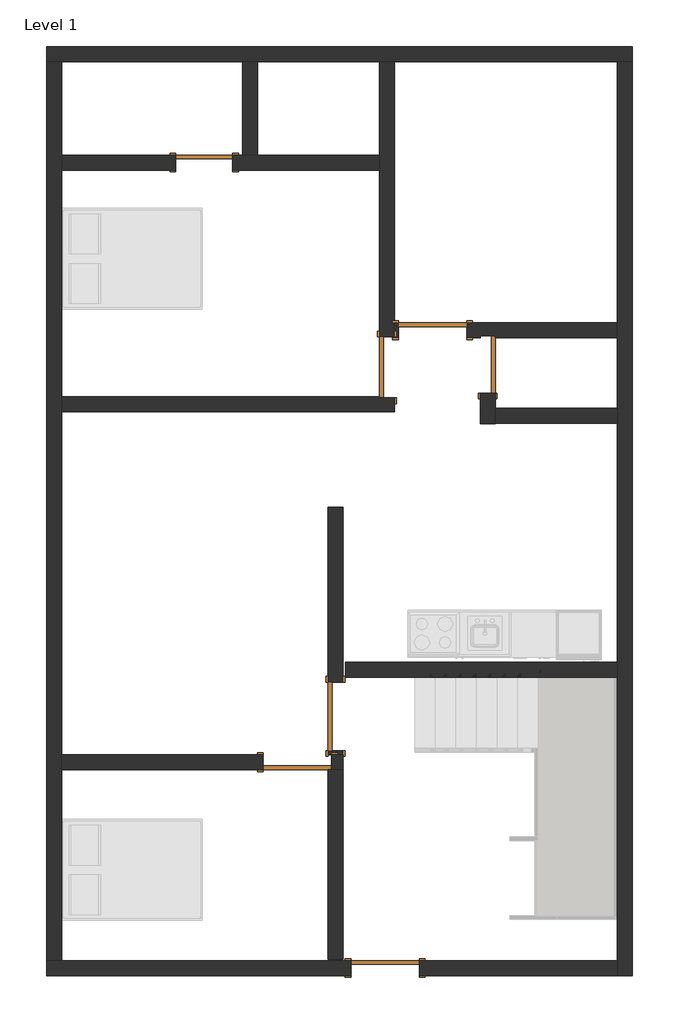
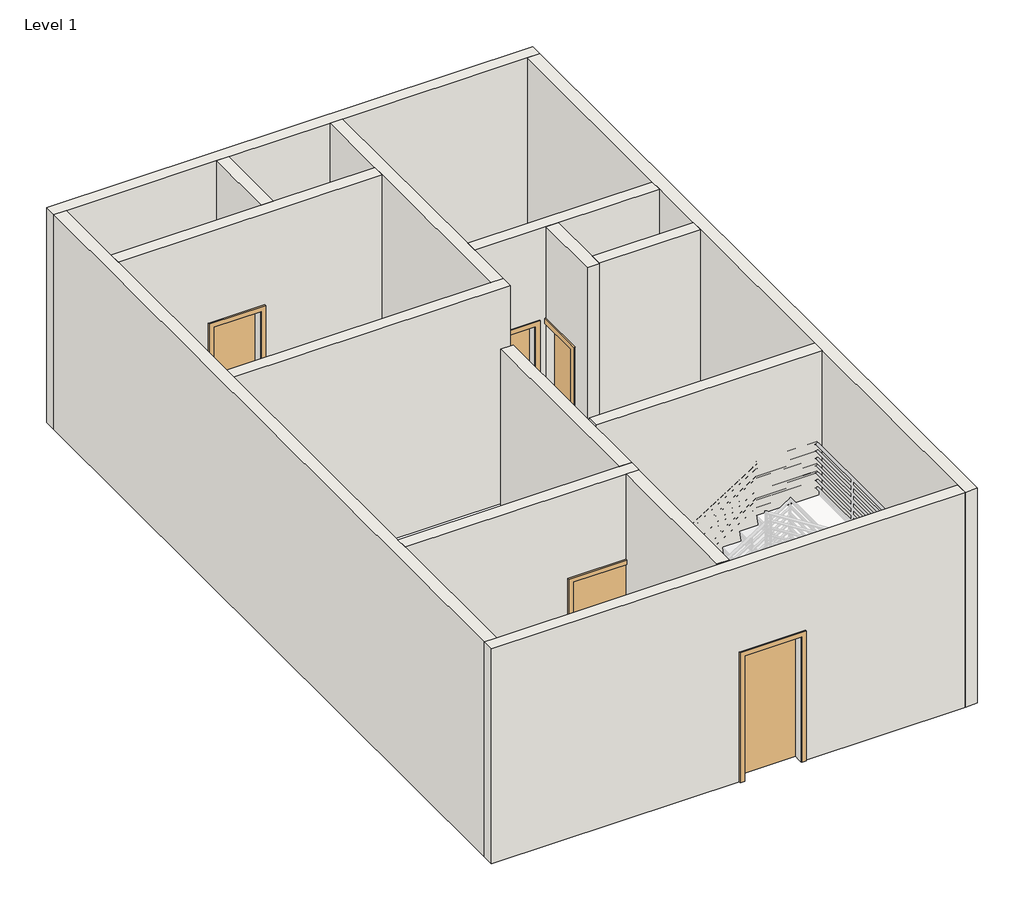
# One storey, part 1 of 4: 15 walls, 7 doors.
"""IFC4 building model written with IfcOpenShell, lengths in millimetres."""

from ifc_helpers import new_model, si_unit, origin, origin_with_axes, place, context, project, spatial, polyline, outline, extrude, faceted_brep, transform, mapped, element, save
from components import m_single_flush_0762_x_2032mm_0c256fab, m_single_flush_0762_x_2032mm_7341a4fb, m_single_flush_0813_x_2134mm_c8a1819b, m_single_flush_0915_x_2032mm_26613924, m_single_flush_0915_x_2134mm_727434cd

model = new_model("IFC4")

# Units and contexts
model_context = context("Model", 3, world=origin())
ifc_project = project(units=[si_unit("LENGTHUNIT", "METRE", prefix="MILLI")], contexts=[model_context])

# Site, building, storey
site = spatial("IfcSite", under=ifc_project)
building = spatial("IfcBuilding", under=site)
storey = spatial("IfcBuildingStorey", under=building, Name="Level 1", Elevation=0.0)

# Doors
placement = place(None, origin())
m_single_flush_0762_x_2032mm_shape = m_single_flush_0762_x_2032mm_0c256fab(model_context)
element("IfcDoor", 1, ObjectType="M_Single-Flush : 0762 x 2032mm", at=placement, inside=storey, context=model_context, shape_type="MappedRepresentation", body=[
    mapped(m_single_flush_0762_x_2032mm_shape, transform((-11550.6689427, 8974.1602653, 0.0), x_axis=(1.0, 0.0, 0.0), y_axis=(0.0, 1.0, 0.0), z_axis=(0.0, 0.0, 1.0))),
])
m_single_flush_0762_x_2032mm_2_shape = m_single_flush_0762_x_2032mm_7341a4fb(model_context)
element("IfcDoor", 2, ObjectType="M_Single-Flush : 0762 x 2032mm", at=placement, inside=storey, context=model_context, shape_type="MappedRepresentation", body=[
    mapped(m_single_flush_0762_x_2032mm_2_shape, transform((-7766.0689427, 6280.1602653, 0.0), x_axis=(0.0, 1.0, 0.0), y_axis=(-1.0, 0.0, 0.0), z_axis=(0.0, 0.0, 1.0))),
])
m_single_flush_0813_x_2134mm_shape = m_single_flush_0813_x_2134mm_c8a1819b(model_context)
element("IfcDoor", 3, ObjectType="M_Single-Flush : 0813 x 2134mm", at=placement, inside=storey, context=model_context, shape_type="MappedRepresentation", body=[
    mapped(m_single_flush_0813_x_2134mm_shape, transform((-9110.6689427, 6242.8602653, 0.0), x_axis=(0.0, -1.0, 0.0), y_axis=(1.0, 0.0, 0.0), z_axis=(0.0, 0.0, 1.0))),
])
m_single_flush_0915_x_2032mm_shape = m_single_flush_0915_x_2032mm_26613924(model_context)
element("IfcDoor", 4, ObjectType="M_Single-Flush : 0915 x 2032mm", at=placement, inside=storey, context=model_context, shape_type="MappedRepresentation", body=[
    mapped(m_single_flush_0915_x_2032mm_shape, transform((-8501.0689427, 6737.3602653, 0.0), x_axis=(-1.0, 0.0, 0.0), y_axis=(0.0, -1.0, 0.0), z_axis=(0.0, 0.0, 1.0))),
])
m_single_flush_0915_x_2134mm_shape = m_single_flush_0915_x_2134mm_727434cd(model_context)
element("IfcDoor", 5, ObjectType="M_Single-Flush : 0915 x 2134mm", at=placement, inside=storey, context=model_context, shape_type="MappedRepresentation", body=[
    mapped(m_single_flush_0915_x_2134mm_shape, transform((-10307.6689427, 976.3602653, 0.0), x_axis=(1.0, 0.0, 0.0), y_axis=(0.0, 1.0, 0.0), z_axis=(0.0, 0.0, 1.0))),
])
element("IfcDoor", 6, ObjectType="M_Single-Flush : 0915 x 2134mm", at=placement, inside=storey, context=model_context, shape_type="MappedRepresentation", body=[
    mapped(m_single_flush_0915_x_2134mm_shape, transform((-9798.0689427, 1585.9602653, 0.0), x_axis=(0.0, -1.0, 0.0), y_axis=(1.0, 0.0, 0.0), z_axis=(0.0, 0.0, 1.0))),
])
element("IfcDoor", 7, ObjectType="M_Single-Flush : 0915 x 2134mm", at=placement, inside=storey, context=model_context, shape_type="MappedRepresentation", body=[
    mapped(m_single_flush_0915_x_2134mm_shape, transform((-9136.0689427, -1770.0397347, 0.0), x_axis=(-1.0, 0.0, 0.0), y_axis=(0.0, -1.0, 0.0), z_axis=(0.0, 0.0, 1.0))),
])

# Walls
element("IfcWall", 8, ObjectType="Generic - 200mm", at=placement, inside=storey, context=model_context, shape_type="Brep", body=[
    faceted_brep([(-13655.6689427, 10321.9602653, 0.0), (-13455.6689427, 10321.9602653, 0.0), (-11041.0689427, 10321.9602653, 0.0), (-10841.0689427, 10321.9602653, 0.0), (-9210.6689427, 10321.9602653, 0.0), (-9010.6689427, 10321.9602653, 0.0), (-6035.6689427, 10321.9602653, 0.0), (-5835.6689427, 10321.9602653, 0.0), (-5835.6689427, 10321.9602653, 3657.6), (-6035.6689427, 10321.9602653, 3657.6), (-9010.6689427, 10321.9602653, 3657.6), (-9210.6689427, 10321.9602653, 3657.6), (-10841.0689427, 10321.9602653, 3657.6), (-11041.0689427, 10321.9602653, 3657.6), (-13455.6689427, 10321.9602653, 3657.6), (-13655.6689427, 10321.9602653, 3657.6), (-13655.6689427, 10521.9602653, 0.0), (-13655.6689427, 10521.9602653, 3657.6), (-5835.6689427, 10521.9602653, 3657.6), (-5835.6689427, 10521.9602653, 0.0)], [[[0, 1, 2, 3, 4, 5, 6, 7, 8, 9, 10, 11, 12, 13, 14, 15]], [[16, 17, 18, 19]], [[7, 6, 5, 4, 3, 2, 1, 0, 16, 19]], [[15, 14, 13, 12, 11, 10, 9, 8, 18, 17]], [[8, 7, 19, 18]], [[0, 15, 17, 16]]]),
])
element("IfcWall", 9, ObjectType="Generic - 200mm", at=placement, inside=storey, context=model_context, shape_type="Brep", body=[
    faceted_brep([(-6035.6689427, 10321.9602653, 0.0), (-6035.6689427, 6837.3602653, 0.0), (-6035.6689427, 6637.3602653, 0.0), (-6035.6689427, 5695.1602653, 0.0), (-6035.6689427, 5495.1602653, 0.0), (-6035.6689427, 2311.9311514, 0.0), (-6035.6689427, 2111.9311514, 0.0), (-6035.6689427, -1670.0397347, 0.0), (-6035.6689427, -1870.0397347, 0.0), (-6035.6689427, -1870.0397347, 3657.6), (-6035.6689427, -1670.0397347, 3657.6), (-6035.6689427, 2111.9311514, 3657.6), (-6035.6689427, 2311.9311514, 3657.6), (-6035.6689427, 5495.1602653, 3657.6), (-6035.6689427, 5695.1602653, 3657.6), (-6035.6689427, 6637.3602653, 3657.6), (-6035.6689427, 6837.3602653, 3657.6), (-6035.6689427, 10321.9602653, 3657.6), (-5835.6689427, 10321.9602653, 0.0), (-5835.6689427, 10321.9602653, 3657.6), (-5835.6689427, -1870.0397347, 3657.6), (-5835.6689427, -1870.0397347, 0.0)], [[[0, 1, 2, 3, 4, 5, 6, 7, 8, 9, 10, 11, 12, 13, 14, 15, 16, 17]], [[18, 19, 20, 21]], [[8, 7, 6, 5, 4, 3, 2, 1, 0, 18, 21]], [[17, 16, 15, 14, 13, 12, 11, 10, 9, 20, 19]], [[0, 17, 19, 18]], [[9, 8, 21, 20]]]),
])
element("IfcWall", 10, ObjectType="Generic - 200mm", at=placement, inside=storey, context=model_context, shape_type="Brep", body=[
    faceted_brep([(-9593.5689427, -1670.0397347, 2134.0), (-9593.5689427, -1670.0397347, 0.0), (-13455.6689427, -1670.0397347, 0.0), (-13655.6689427, -1670.0397347, 0.0), (-13655.6689427, -1670.0397347, 3657.6), (-13455.6689427, -1670.0397347, 3657.6), (-6035.6689427, -1670.0397347, 3657.6), (-6035.6689427, -1670.0397347, 0.0), (-8678.5689427, -1670.0397347, 0.0), (-8678.5689427, -1670.0397347, 2134.0), (-13655.6689427, -1870.0397347, 0.0), (-9593.5689427, -1870.0397347, 0.0), (-9593.5689427, -1870.0397347, 2134.0), (-8678.5689427, -1870.0397347, 2134.0), (-8678.5689427, -1870.0397347, 0.0), (-6035.6689427, -1870.0397347, 0.0), (-6035.6689427, -1870.0397347, 3657.6), (-13655.6689427, -1870.0397347, 3657.6)], [[[0, 1, 2, 3, 4, 5, 6, 7, 8, 9]], [[10, 11, 12, 13, 14, 15, 16, 17]], [[8, 7, 15, 14]], [[3, 2, 1, 11, 10]], [[6, 5, 4, 17, 16]], [[7, 6, 16, 15]], [[4, 3, 10, 17]], [[12, 11, 1, 0]], [[13, 12, 0, 9]], [[14, 13, 9, 8]]]),
])
element("IfcWall", 11, ObjectType="Generic - 200mm", at=placement, inside=storey, context=model_context, shape_type="Brep", body=[
    faceted_brep([(-13455.6689427, -1670.0397347, 0.0), (-13455.6689427, 876.3602653, 0.0), (-13455.6689427, 1076.3602653, 0.0), (-13455.6689427, 5648.3602653, 0.0), (-13455.6689427, 5848.3602653, 0.0), (-13455.6689427, 8874.1602653, 0.0), (-13455.6689427, 9074.1602653, 0.0), (-13455.6689427, 10321.9602653, 0.0), (-13455.6689427, 10321.9602653, 3657.6), (-13455.6689427, 9074.1602653, 3657.6), (-13455.6689427, 8874.1602653, 3657.6), (-13455.6689427, 5848.3602653, 3657.6), (-13455.6689427, 5648.3602653, 3657.6), (-13455.6689427, 1076.3602653, 3657.6), (-13455.6689427, 876.3602653, 3657.6), (-13455.6689427, -1670.0397347, 3657.6), (-13655.6689427, -1670.0397347, 0.0), (-13655.6689427, -1670.0397347, 3657.6), (-13655.6689427, 10321.9602653, 3657.6), (-13655.6689427, 10321.9602653, 0.0)], [[[0, 1, 2, 3, 4, 5, 6, 7, 8, 9, 10, 11, 12, 13, 14, 15]], [[16, 17, 18, 19]], [[7, 6, 5, 4, 3, 2, 1, 0, 16, 19]], [[15, 14, 13, 12, 11, 10, 9, 8, 18, 17]], [[8, 7, 19, 18]], [[0, 15, 17, 16]]]),
])
element("IfcWall", 12, ObjectType="Generic - 200mm", at=placement, inside=storey, context=model_context, shape_type="Brep", body=[
    faceted_brep([(-11169.6689427, 8874.1602653, 2032.0), (-11169.6689427, 8874.1602653, 0.0), (-9210.6689427, 8874.1602653, 0.0), (-9210.6689427, 8874.1602653, 3657.6), (-13455.6689427, 8874.1602653, 3657.6), (-13455.6689427, 8874.1602653, 0.0), (-11931.6689427, 8874.1602653, 0.0), (-11931.6689427, 8874.1602653, 2032.0), (-9210.6689427, 9074.1602653, 0.0), (-10841.0689427, 9074.1602653, 0.0), (-11041.0689427, 9074.1602653, 0.0), (-11169.6689427, 9074.1602653, 0.0), (-11169.6689427, 9074.1602653, 2032.0), (-11931.6689427, 9074.1602653, 2032.0), (-11931.6689427, 9074.1602653, 0.0), (-13455.6689427, 9074.1602653, 0.0), (-13455.6689427, 9074.1602653, 3657.6), (-11041.0689427, 9074.1602653, 3657.6), (-10841.0689427, 9074.1602653, 3657.6), (-9210.6689427, 9074.1602653, 3657.6)], [[[0, 1, 2, 3, 4, 5, 6, 7]], [[8, 9, 10, 11, 12, 13, 14, 15, 16, 17, 18, 19]], [[6, 5, 15, 14]], [[2, 1, 11, 10, 9, 8]], [[4, 3, 19, 18, 17, 16]], [[5, 4, 16, 15]], [[3, 2, 8, 19]], [[12, 11, 1, 0]], [[13, 12, 0, 7]], [[14, 13, 7, 6]]]),
])
element("IfcWall", 13, ObjectType="Generic - 200mm", at=placement, inside=storey, context=model_context, shape_type="SweptSolid", body=[
    extrude(outline(polyline([(-10841.0689427, 10321.9602653), (-10841.0689427, 9074.1602653), (-11041.0689427, 9074.1602653), (-11041.0689427, 10321.9602653), (-10841.0689427, 10321.9602653)])), origin_with_axes(), (0.0, 0.0, 1.0), 3657.6),
])
element("IfcWall", 14, ObjectType="Generic - 200mm", at=placement, inside=storey, context=model_context, shape_type="Brep", body=[
    faceted_brep([(-9010.6689427, 6837.3602653, 3657.6), (-6035.6689427, 6837.3602653, 3657.6), (-6035.6689427, 6837.3602653, 0.0), (-8043.5689427, 6837.3602653, 0.0), (-8043.5689427, 6837.3602653, 2032.0), (-8958.5689427, 6837.3602653, 2032.0), (-8958.5689427, 6837.3602653, 0.0), (-9010.6689427, 6837.3602653, 0.0), (-6035.6689427, 6637.3602653, 3657.6), (-7666.0689427, 6637.3602653, 3657.6), (-7866.0689427, 6637.3602653, 3657.6), (-9010.6689427, 6637.3602653, 3657.6), (-9010.6689427, 6637.3602653, 0.0), (-8958.5689427, 6637.3602653, 0.0), (-8958.5689427, 6637.3602653, 2032.0), (-8043.5689427, 6637.3602653, 2032.0), (-8043.5689427, 6637.3602653, 0.0), (-7866.0689427, 6637.3602653, 0.0), (-7866.0689427, 6637.3602653, 2032.0), (-7666.0689427, 6637.3602653, 2032.0), (-7666.0689427, 6637.3602653, 0.0), (-6035.6689427, 6637.3602653, 0.0), (-7666.0689427, 6661.1602653, 0.0), (-7866.0689427, 6661.1602653, 0.0), (-9010.6689427, 6649.3602653, 0.0), (-7666.0689427, 6661.1602653, 2032.0), (-7866.0689427, 6661.1602653, 2032.0)], [[[0, 1, 2, 3, 4, 5, 6, 7]], [[8, 9, 10, 11, 12, 13, 14, 15, 16, 17, 18, 19, 20, 21]], [[2, 21, 20, 22, 23, 17, 16, 3]], [[12, 24, 7, 6, 13]], [[1, 0, 11, 10, 9, 8]], [[0, 7, 24, 12, 11]], [[2, 1, 8, 21]], [[14, 13, 6, 5]], [[15, 14, 5, 4]], [[16, 15, 4, 3]], [[25, 22, 20, 19]], [[23, 26, 18, 17]], [[22, 25, 26, 23]], [[26, 25, 19, 18]]]),
])
element("IfcWall", 15, ObjectType="Generic - 200mm", at=placement, inside=storey, context=model_context, shape_type="Brep", body=[
    faceted_brep([(-9010.6689427, 10321.9602653, 3657.6), (-9010.6689427, 6837.3602653, 3657.6), (-9010.6689427, 6637.3602653, 3657.6), (-9010.6689427, 5848.3602653, 3657.6), (-9010.6689427, 5848.3602653, 2134.0), (-9010.6689427, 6649.3602653, 2134.0), (-9010.6689427, 6649.3602653, 0.0), (-9010.6689427, 6837.3602653, 0.0), (-9010.6689427, 10321.9602653, 0.0), (-9210.6689427, 5848.3602653, 3657.6), (-9210.6689427, 8874.1602653, 3657.6), (-9210.6689427, 9074.1602653, 3657.6), (-9210.6689427, 10321.9602653, 3657.6), (-9210.6689427, 10321.9602653, 0.0), (-9210.6689427, 9074.1602653, 0.0), (-9210.6689427, 8874.1602653, 0.0), (-9210.6689427, 6649.3602653, 0.0), (-9210.6689427, 6649.3602653, 2134.0), (-9210.6689427, 5848.3602653, 2134.0)], [[[0, 1, 2, 3, 4, 5, 6, 7, 8]], [[9, 10, 11, 12, 13, 14, 15, 16, 17, 18]], [[13, 8, 7, 6, 16, 15, 14]], [[3, 2, 1, 0, 12, 11, 10, 9]], [[0, 8, 13, 12]], [[3, 9, 18, 4]], [[17, 5, 4, 18]], [[5, 17, 16, 6]]]),
])
element("IfcWall", 16, ObjectType="Generic - 200mm", at=placement, inside=storey, context=model_context, shape_type="Brep", body=[
    faceted_brep([(-13455.6689427, 5648.3602653, 0.0), (-9010.6689427, 5648.3602653, 0.0), (-9010.6689427, 5648.3602653, 3657.6), (-13455.6689427, 5648.3602653, 3657.6), (-13455.6689427, 5848.3602653, 3657.6), (-9210.6689427, 5848.3602653, 3657.6), (-9010.6689427, 5848.3602653, 3657.6), (-9010.6689427, 5848.3602653, 2134.0), (-9210.6689427, 5848.3602653, 2134.0), (-9210.6689427, 5848.3602653, 0.0), (-13455.6689427, 5848.3602653, 0.0), (-9210.6689427, 5836.3602653, 0.0), (-9010.6689427, 5836.3602653, 0.0), (-9010.6689427, 5836.3602653, 2134.0), (-9210.6689427, 5836.3602653, 2134.0)], [[[0, 1, 2, 3]], [[4, 5, 6, 7, 8, 9, 10]], [[1, 0, 10, 9, 11, 12]], [[3, 2, 6, 5, 4]], [[0, 3, 4, 10]], [[2, 1, 12, 13, 7, 6]], [[14, 11, 9, 8]], [[11, 14, 13, 12]], [[13, 14, 8, 7]]]),
])
element("IfcWall", 17, ObjectType="Generic - 200mm", at=placement, inside=storey, context=model_context, shape_type="Brep", body=[
    faceted_brep([(-7666.0689427, 6637.3602653, 3657.6), (-7666.0689427, 5695.1602653, 3657.6), (-7666.0689427, 5495.1602653, 3657.6), (-7666.0689427, 5491.1602653, 3657.6), (-7666.0689427, 5491.1602653, 0.0), (-7666.0689427, 5495.1602653, 0.0), (-7666.0689427, 5695.1602653, 0.0), (-7666.0689427, 5899.1602653, 0.0), (-7666.0689427, 5899.1602653, 2032.0), (-7666.0689427, 6637.3602653, 2032.0), (-7866.0689427, 5491.1602653, 3657.6), (-7866.0689427, 6637.3602653, 3657.6), (-7866.0689427, 6637.3602653, 2032.0), (-7866.0689427, 5899.1602653, 2032.0), (-7866.0689427, 5899.1602653, 0.0), (-7866.0689427, 5491.1602653, 0.0)], [[[0, 1, 2, 3, 4, 5, 6, 7, 8, 9]], [[10, 11, 12, 13, 14, 15]], [[4, 15, 14, 7, 6, 5]], [[3, 2, 1, 0, 11, 10]], [[4, 3, 10, 15]], [[11, 0, 9, 12]], [[8, 13, 12, 9]], [[13, 8, 7, 14]]]),
])
element("IfcWall", 18, ObjectType="Generic - 200mm", at=placement, inside=storey, context=model_context, shape_type="Brep", body=[
    faceted_brep([(-9698.0689427, 876.3602653, 3657.6), (-9701.1689427, 876.3602653, 3657.6), (-9901.1689427, 876.3602653, 3657.6), (-13455.6689427, 876.3602653, 3657.6), (-13455.6689427, 876.3602653, 0.0), (-10765.1689427, 876.3602653, 0.0), (-10765.1689427, 876.3602653, 2134.0), (-9850.1689427, 876.3602653, 2134.0), (-9850.1689427, 876.3602653, 0.0), (-9701.1689427, 876.3602653, 0.0), (-9698.0689427, 876.3602653, 0.0), (-13455.6689427, 1076.3602653, 3657.6), (-9898.0689427, 1076.3602653, 3657.6), (-9698.0689427, 1076.3602653, 3657.6), (-9698.0689427, 1076.3602653, 0.0), (-9850.1689427, 1076.3602653, 0.0), (-9850.1689427, 1076.3602653, 2134.0), (-10765.1689427, 1076.3602653, 2134.0), (-10765.1689427, 1076.3602653, 0.0), (-13455.6689427, 1076.3602653, 0.0)], [[[0, 1, 2, 3, 4, 5, 6, 7, 8, 9, 10]], [[11, 12, 13, 14, 15, 16, 17, 18, 19]], [[4, 19, 18, 5]], [[14, 10, 9, 8, 15]], [[3, 2, 1, 0, 13, 12, 11]], [[4, 3, 11, 19]], [[7, 16, 15, 8]], [[17, 6, 5, 18]], [[6, 17, 16, 7]], [[0, 10, 14, 13]]]),
])
element("IfcWall", 19, ObjectType="Generic - 200mm", at=placement, inside=storey, context=model_context, shape_type="SweptSolid", body=[
    extrude(outline(polyline([(-6035.6689427, 5495.1602653), (-7666.0689427, 5495.1602653), (-7666.0689427, 5695.1602653), (-6035.6689427, 5695.1602653), (-6035.6689427, 5495.1602653)])), origin_with_axes(), (0.0, 0.0, 1.0), 3657.6),
])
element("IfcWall", 20, ObjectType="Generic - 200mm", at=placement, inside=storey, context=model_context, shape_type="Brep", body=[
    faceted_brep([(-9898.0689427, 1128.4602653, 2134.0), (-9898.0689427, 1128.4602653, 0.0), (-9898.0689427, 1076.3602653, 0.0), (-9898.0689427, 1076.3602653, 3657.6), (-9898.0689427, 4375.9602653, 3657.6), (-9898.0689427, 4375.9602653, 0.0), (-9898.0689427, 2043.4602653, 0.0), (-9898.0689427, 2043.4602653, 2134.0), (-9698.0689427, 1076.3602653, 0.0), (-9698.0689427, 1128.4602653, 0.0), (-9698.0689427, 1128.4602653, 2134.0), (-9698.0689427, 2043.4602653, 2134.0), (-9698.0689427, 2043.4602653, 0.0), (-9698.0689427, 4375.9602653, 0.0), (-9698.0689427, 4375.9602653, 3657.6), (-9698.0689427, 1076.3602653, 3657.6), (-9850.1689427, 1076.3602653, 0.0)], [[[0, 1, 2, 3, 4, 5, 6, 7]], [[8, 9, 10, 11, 12, 13, 14, 15]], [[6, 5, 13, 12]], [[2, 1, 9, 8, 16]], [[4, 3, 15, 14]], [[5, 4, 14, 13]], [[3, 2, 16, 8, 15]], [[10, 9, 1, 0]], [[11, 10, 0, 7]], [[12, 11, 7, 6]]]),
])
element("IfcWall", 21, ObjectType="Generic - 200mm", at=placement, inside=storey, context=model_context, shape_type="SweptSolid", body=[
    extrude(outline(polyline([(-9901.1689427, -1651.2909018), (-9901.1689427, 876.3602653), (-9701.1689427, 876.3602653), (-9701.1689427, -1651.2909018), (-9901.1689427, -1651.2909018)])), origin_with_axes(), (0.0, 0.0, 1.0), 3657.6),
])
element("IfcWall", 22, ObjectType="Generic - 200mm", at=placement, inside=storey, context=model_context, shape_type="SweptSolid", body=[
    extrude(outline(polyline([(-9667.8689427, 2311.9311514), (-6035.6689427, 2311.9311514), (-6035.6689427, 2111.9311514), (-9667.8689427, 2111.9311514), (-9667.8689427, 2311.9311514)])), origin_with_axes(), (0.0, 0.0, 1.0), 3657.6),
])

save(model, "model.ifc")

# Revit data of these elements
# Type "M_Single-Flush : 0762 x 2032mm"
#   Type Mark = "19"
#   Thickness = 51 mm
#   Height = 2032 mm
#   Trim Projection Ext = 25 mm
#   Trim Projection Int = 25 mm
#   Trim Width = 76 mm
#   Width = 762 mm
#   Door Material = Door - Panel
#   Frame Material = Door - Frame
#   Function = (empty or 0)
#   Wall Closure = (empty or 0)
# Type "M_Single-Flush : 0813 x 2134mm"
#   Type Mark = "17"
#   Thickness = 51 mm
#   Height = 2134 mm
#   Trim Projection Ext = 25 mm
#   Trim Projection Int = 25 mm
#   Trim Width = 76 mm
#   Width = 813 mm
#   Door Material = Door - Panel
#   Frame Material = Door - Frame
#   Function = (empty or 0)
#   Wall Closure = (empty or 0)
# Type "M_Single-Flush : 0915 x 2032mm"
#   Type Mark = "20"
#   Thickness = 51 mm
#   Height = 2032 mm
#   Trim Projection Ext = 25 mm
#   Trim Projection Int = 25 mm
#   Trim Width = 76 mm
#   Width = 915 mm
#   Door Material = Door - Panel
#   Frame Material = Door - Frame
#   Function = (empty or 0)
#   Wall Closure = (empty or 0)
# Type "M_Single-Flush : 0915 x 2134mm"
#   Type Mark = "15"
#   Thickness = 51 mm
#   Height = 2134 mm
#   Trim Projection Ext = 25 mm
#   Trim Projection Int = 25 mm
#   Trim Width = 76 mm
#   Width = 915 mm
#   Door Material = Door - Panel
#   Frame Material = Door - Frame
#   Function = (empty or 0)
#   Wall Closure = (empty or 0)
# Type "Generic - 200mm"
#   Layers, outside or top first: 200 mm no material (function 1)
# Elements 1, 2 (IfcDoor, "M_Single-Flush : 0762 x 2032mm")
#   Phase Created = New Construction
#   Materials on its faces: "Door - Frame", "Door - Panel"
# Element 3 (IfcDoor, "M_Single-Flush : 0813 x 2134mm")
#   Phase Created = New Construction
#   Materials on its faces: "Door - Frame", "Door - Panel"
# Element 4 (IfcDoor, "M_Single-Flush : 0915 x 2032mm")
#   Phase Created = New Construction
#   Materials on its faces: "Door - Frame", "Door - Panel"
# Elements 5, 6, 7 (IfcDoor, "M_Single-Flush : 0915 x 2134mm")
#   Phase Created = New Construction
#   Materials on its faces: "Door - Frame", "Door - Panel"
# Elements 8, 9, 10, 11, 12, 13, 14, 15, 16, 17, 18, 19, 20, 21, 22 (IfcWall, "Generic - 200mm")
#   Top Offset = 0 mm
#   Base Offset = 0 mm
#   Unconnected Height = 3657.6 mm
#   wall height = 3657.6 mm
#   Phase Created = New Construction
#   Base Constraint = Level 1
#   Materials on its faces: "Default Wall"
# Materials
#   "Door - Panel": class "Wood", colour RGB 114 82 51, transparency 0
#   "Door - Frame": colour RGB 153 76 43, transparency 0
#   "Default Wall": colour RGB 80 80 80, transparency 0
